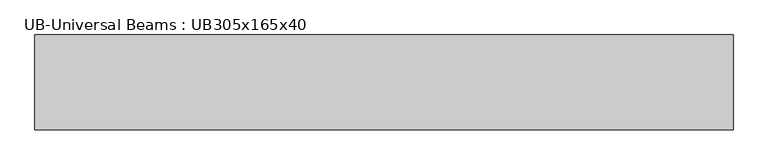
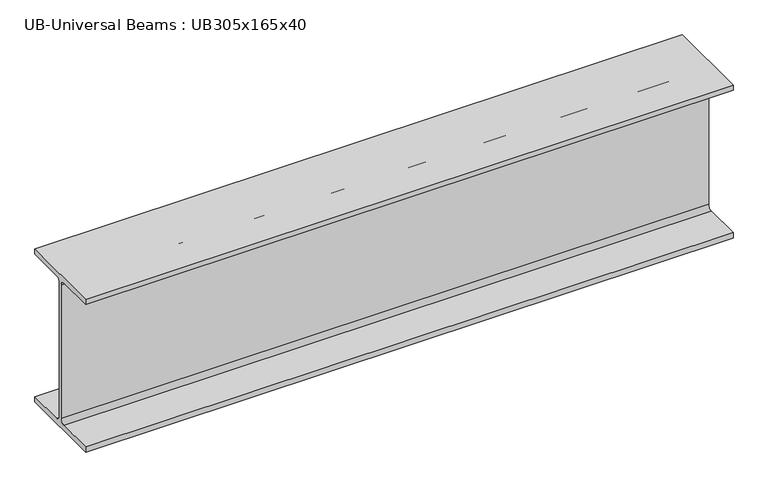
"""IFC4 building model written with IfcOpenShell, lengths in millimetres: beam geometry, UB-Universal Beams : UB305x165x40."""

from ifc_helpers import new_model, si_unit, point, frame, frame_2d, origin, place, context, project, spatial, polyline, circle_curve, trimmed, segment, composite_curve, outline, extrude, source, transform, mapped, element, save


def ub_universal_beams_ub305x165x40_555319cc(model_context):
    return source(origin(), model_context, "Body", "SweptSolid", [
        extrude(outline(composite_curve([segment(polyline([(82.5, -141.5), (82.5, -151.7), (-82.5, -151.7), (-82.5, -141.5), (-11.9, -141.5)]), True, "CONTINUOUS"), segment(trimmed(circle_curve(frame_2d((-11.9, -132.6)), 8.9), [point((-11.9, -141.5))], [point((-3.0, -132.6))], True, "CARTESIAN"), True, "CONTINUOUS"), segment(polyline([(-3.0, -132.6), (-3.0, 132.6)]), True, "CONTINUOUS"), segment(trimmed(circle_curve(frame_2d((-11.9, 132.6)), 8.9), [point((-3.0, 132.6))], [point((-11.9, 141.5))], True, "CARTESIAN"), True, "CONTINUOUS"), segment(polyline([(-11.9, 141.5), (-82.5, 141.5), (-82.5, 151.7), (82.5, 151.7), (82.5, 141.5), (11.9, 141.5)]), True, "CONTINUOUS"), segment(trimmed(circle_curve(frame_2d((11.9, 132.6)), 8.9), [point((11.9, 141.5))], [point((3.0, 132.6))], True, "CARTESIAN"), True, "CONTINUOUS"), segment(polyline([(3.0, 132.6), (3.0, -132.6)]), True, "CONTINUOUS"), segment(trimmed(circle_curve(frame_2d((11.9, -132.6)), 8.9), [point((3.0, -132.6))], [point((11.9, -141.5))], True, "CARTESIAN"), True, "CONTINUOUS"), segment(polyline([(11.9, -141.5), (82.5, -141.5)]), True, "CONTINUOUS")], self_intersect=False)), frame((-391.7, 0.0, 0.0), z_axis=(1.0, 0.0, 0.0), x_axis=(0.0, 1.0, 0.0)), (0.0, 0.0, 1.0), 1215.8),
    ])


if __name__ == "__main__":
    model = new_model("IFC4")
    model_context = context("Model", 3, world=origin())
    ifc_project = project(units=[si_unit("LENGTHUNIT", "METRE", prefix="MILLI")], contexts=[model_context])
    site = spatial("IfcSite", under=ifc_project)
    building = spatial("IfcBuilding", under=site)
    placement = place(None, origin())
    ub_universal_beams_ub305x165x40_shape = ub_universal_beams_ub305x165x40_555319cc(model_context)
    element("IfcBeam", 1, ObjectType="UB-Universal Beams : UB305x165x40", at=placement, inside=building, context=model_context, shape_type="MappedRepresentation", body=[
        mapped(ub_universal_beams_ub305x165x40_shape, transform((0.0, 0.0, 0.0), x_axis=(1.0, 0.0, 0.0), y_axis=(0.0, 1.0, 0.0), z_axis=(0.0, 0.0, 1.0))),
    ])
    save(model, "model.ifc")

# Revit data of these elements
# Type "UB-Universal Beams : UB305x165x40"
#   Section Name Key = "UB305X165X40"
#   Width = 16.5 cm
#   Web Thickness = 0.6 cm
#   Web Fillet = 0.89 cm
#   Warping Constant = 164000.0 cm⁶
#   Torsional Moment of Inertia = 14.70 cm⁴
#   Section Area = 51.3 cm²
#   Plastic Modulus weak axis = 142.0 cm³
#   Plastic Modulus strong axis = 623.0 cm³
#   Nominal Weight = 40.2999 kgf/m
#   Moment of Inertia weak axis = 764.00 cm⁴
#   Moment of Inertia strong axis = 8503.00 cm⁴
#   Height = 30.34 cm
#   Flange Thickness = 1.02 cm
#   Elastic Modulus weak axis = 92.6 cm³
#   Elastic Modulus strong axis = 560.0 cm³
#   Centroid Vertical = 15.17 cm
#   Centroid Horizontal = 8.25 cm
#   Bolt Spacing = 9.0 cm
#   Length [instance default] = 1500 mm
#   Structural Material [instance default] = Metal - Steel 43-275
#   Type Comments = ""
#   Assembly Code = ""
# Element 1 (IfcBeam, "UB-Universal Beams : UB305x165x40")
#   Materials on its faces: "Metal - Steel 43-275"
# Materials
#   "Metal - Steel 43-275": class "Metal", colour RGB 247 247 247, transparency 0, Cost = 0
